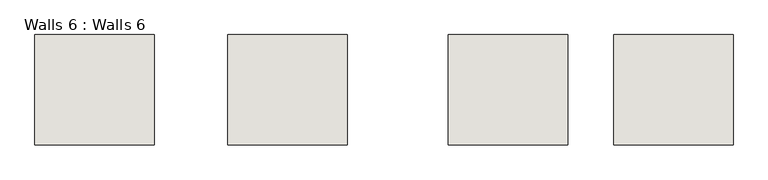
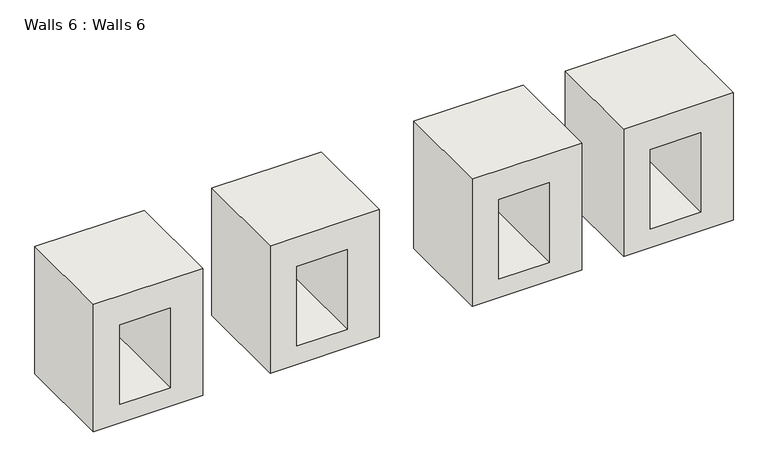
"""IFC4 building model written with IfcOpenShell, lengths in millimetres: wall geometry, Walls 6 : Walls 6."""

from ifc_helpers import new_model, si_unit, frame, origin, place, context, project, spatial, polyline, outline, extrude, source, transform, mapped, element, save


def walls_6_walls_6_a828669c(model_context):
    return source(origin(), model_context, "Body", "SweptSolid", [
        extrude(outline(polyline([(2359.9469476, -9350.1407032), (2359.9469476, -9680.3407032), (1953.5469476, -9680.3407032), (1953.5469476, -9350.1407032), (2359.9469476, -9350.1407032)]), holes=[polyline([(2266.5962254, -9447.3706829), (2012.5962254, -9447.3706829), (2012.5962254, -9599.7706829), (2266.5962254, -9599.7706829), (2266.5962254, -9447.3706829)])]), frame((0.0, 3351.3956099, 0.0), z_axis=(0.0, 1.0, 0.0), x_axis=(0.0, 0.0, 1.0)), (0.0, 0.0, 1.0), 304.8),
        extrude(outline(polyline([(2359.9469476, -8816.7407032), (2359.9469476, -9146.9407032), (1953.5469476, -9146.9407032), (1953.5469476, -8816.7407032), (2359.9469476, -8816.7407032)]), holes=[polyline([(2266.5962254, -8913.9706829), (2012.5962254, -8913.9706829), (2012.5962254, -9066.3706829), (2266.5962254, -9066.3706829), (2266.5962254, -8913.9706829)])]), frame((0.0, 3351.3956099, 0.0), z_axis=(0.0, 1.0, 0.0), x_axis=(0.0, 0.0, 1.0)), (0.0, 0.0, 1.0), 304.8),
        extrude(outline(polyline([(2359.9469476, -8207.1407032), (2359.9469476, -8537.3407032), (1953.5469476, -8537.3407032), (1953.5469476, -8207.1407032), (2359.9469476, -8207.1407032)]), holes=[polyline([(2266.5962254, -8304.3706829), (2012.5962254, -8304.3706829), (2012.5962254, -8456.7706829), (2266.5962254, -8456.7706829), (2266.5962254, -8304.3706829)])]), frame((0.0, 3351.3956099, 0.0), z_axis=(0.0, 1.0, 0.0), x_axis=(0.0, 0.0, 1.0)), (0.0, 0.0, 1.0), 304.8),
        extrude(outline(polyline([(2359.9469476, -7749.9407032), (2359.9469476, -8080.1407032), (1953.5469476, -8080.1407032), (1953.5469476, -7749.9407032), (2359.9469476, -7749.9407032)]), holes=[polyline([(2266.5962254, -7847.1706829), (2012.5962254, -7847.1706829), (2012.5962254, -7999.5706829), (2266.5962254, -7999.5706829), (2266.5962254, -7847.1706829)])]), frame((0.0, 3351.3956099, 0.0), z_axis=(0.0, 1.0, 0.0), x_axis=(0.0, 0.0, 1.0)), (0.0, 0.0, 1.0), 304.8),
    ])


if __name__ == "__main__":
    model = new_model("IFC4")
    model_context = context("Model", 3, world=origin())
    ifc_project = project(units=[si_unit("LENGTHUNIT", "METRE", prefix="MILLI")], contexts=[model_context])
    site = spatial("IfcSite", under=ifc_project)
    building = spatial("IfcBuilding", under=site)
    placement = place(None, origin())
    walls_6_walls_6_shape = walls_6_walls_6_a828669c(model_context)
    element("IfcWall", 1, ObjectType="Walls 6 : Walls 6", at=placement, inside=building, context=model_context, shape_type="MappedRepresentation", body=[
        mapped(walls_6_walls_6_shape, transform((0.0, 0.0, 0.0), x_axis=(1.0, 0.0, 0.0), y_axis=(0.0, 1.0, 0.0), z_axis=(0.0, 0.0, 1.0))),
    ])
    save(model, "model.ifc")

# Revit data of these elements
# Element 1 (IfcWall, "Walls 6 : Walls 6")
#   Materials on its faces: "Default Wall"
# Materials
#   "Default Wall": colour RGB 80 80 80, transparency 0
